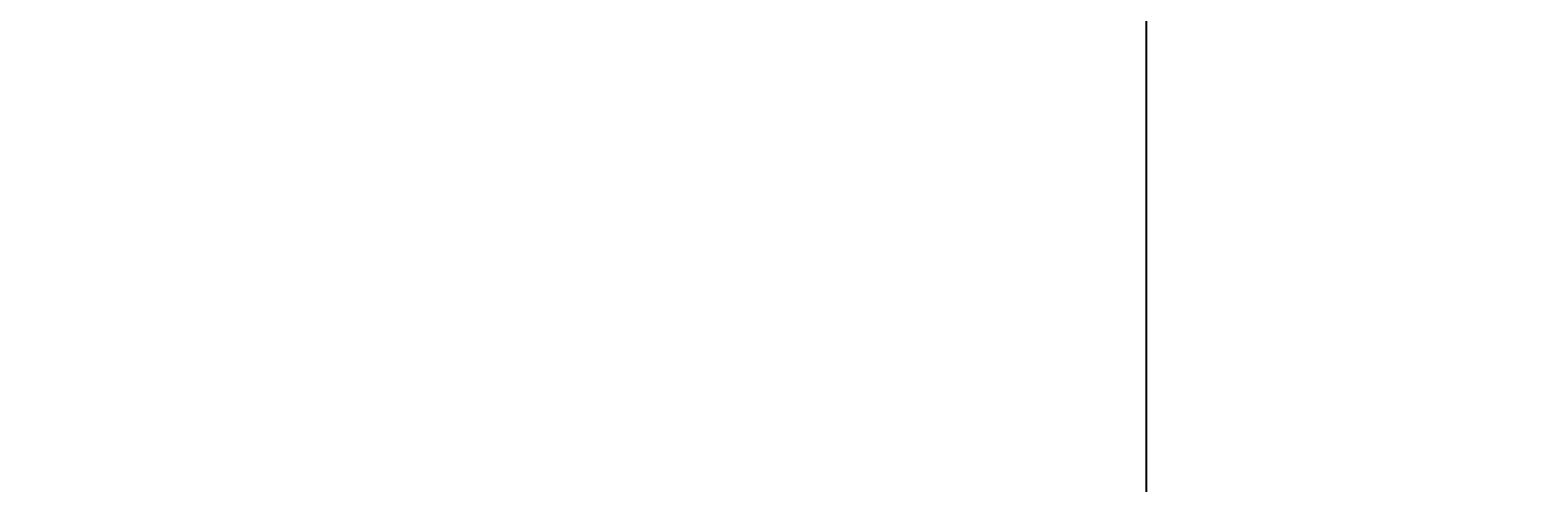
# Model space of a CAD drawing. Units: inches. Extents: x -301 to 715, y -607 to 364.
# Tile 15 of 141: x 18 to 59, y -499 to -486. Entities that reach past the tile are written whole.
import ezdxf

# ---------------------------------------------------------------- set-up
doc = ezdxf.new("R2010")
doc.units = ezdxf.units.IN
doc.header["$MEASUREMENT"] = 0
doc.layers.add('A-ANNO-DIMS', color=2, linetype='Continuous', lineweight=18)
doc.styles.get("Standard").update_dxf_attribs({"font": 'arial.ttf'})
doc.dimstyles.get("Standard").update_dxf_attribs({"dimtxt": 0.18, "dimasz": 0.18, "dimexe": 0.18, "dimexo": 0.0625, "dimgap": 0.09, "dimtad": 0, "dimtih": 1, "dimtoh": 1, "dimdec": 1, "dimzin": 0, "dimdsep": 46, "dimlunit": 4, "dimtxsty": 'Standard', "dimcen": 0.09, "dimclrd": 3, "dimclre": 4, "dimclrt": 6, "dimadec": 0, "dimazin": 0, "dimtfac": 1, "dimtdec": 1, "dimtofl": 0, "dimtmove": 0, "dimatfit": 3, "dimfxl": 1, "dimtfill": 2, "dimtfillclr": 51, "dimtolj": 1, "dimtzin": 0, "dimarcsym": 0})

# ---------------------------------------------------------------- blocks, each defined once
blk = doc.blocks.new('*D176')
at = {"layer": 'A-ANNO-DIMS', "color": 4, "lineweight": -2, "transparency": 16777216}
for p, q in [((148.28, -324.477), (215.605, -324.477)), ((-15.22, -540.477), (215.605, -540.477))]:
    blk.add_line(p, q, dxfattribs=at)
at = {"layer": 'A-ANNO-DIMS', "color": 3, "lineweight": -2, "transparency": 16777216}
for p, q in [((215.425, -324.657), (215.425, -432.296)), ((215.425, -540.297), (215.425, -432.659))]:
    blk.add_line(p, q, dxfattribs=at)
at = {"layer": 'A-ANNO-DIMS', "color": 3, "transparency": 16777216}
for points in [[(215.395, -324.657), (215.455, -324.657), (215.425, -324.477)], [(215.395, -540.297), (215.455, -540.297), (215.425, -540.477)]]:
    blk.add_solid(points, dxfattribs=at)
at = {"layer": 'Defpoints', "color": 0, "transparency": 16777216}
for p in [(148.218, -324.477), (-15.282, -540.477), (215.425, -540.477)]:
    blk.add_point(p, dxfattribs=at)
at = {"layer": 'A-ANNO-DIMS', "color": 6, "transparency": 16777216, "insert": (215.425, -432.477), "char_height": 0.18, "attachment_point": 5, "bg_fill": 1, "box_fill_scale": 1.25, "bg_fill_color": 51, "bg_fill_transparency": 0}
blk.add_mtext('\\A1;18\'-0"', dxfattribs=at)
blk = doc.blocks.new('*D181')
at = {"layer": 'A-ANNO-DIMS', "color": 4, "lineweight": -2, "transparency": 16777216}
for p, q in [((48.468, -433.54), (48.468, -573.809)), ((12.718, -463.54), (12.718, -573.809))]:
    blk.add_line(p, q, dxfattribs=at)
at = {"layer": 'A-ANNO-DIMS', "color": 3, "lineweight": -2, "transparency": 16777216}
for p, q in [((12.898, -573.629), (30.264, -573.629)), ((48.288, -573.629), (30.922, -573.629))]:
    blk.add_line(p, q, dxfattribs=at)
at = {"layer": 'A-ANNO-DIMS', "color": 3, "transparency": 16777216}
for points in [[(12.898, -573.599), (12.898, -573.659), (12.718, -573.629)], [(48.288, -573.599), (48.288, -573.659), (48.468, -573.629)]]:
    blk.add_solid(points, dxfattribs=at)
at = {"layer": 'Defpoints', "color": 0, "transparency": 16777216}
for p in [(48.468, -433.477), (12.718, -463.477), (48.468, -573.629)]:
    blk.add_point(p, dxfattribs=at)
at = {"layer": 'A-ANNO-DIMS', "color": 6, "transparency": 16777216, "insert": (30.593, -573.629), "char_height": 0.18, "attachment_point": 5, "bg_fill": 1, "box_fill_scale": 1.25, "bg_fill_color": 51, "bg_fill_transparency": 0}
blk.add_mtext('\\A1;3\'-0"', dxfattribs=at)
blk = doc.blocks.new('*D190')
at = {"layer": 'A-ANNO-DIMS', "color": 4, "lineweight": -2, "transparency": 16777216}
for p, q in [((129.193, -481.477), (-266.112, -481.477)), ((124.193, -511.477), (-266.112, -511.477))]:
    blk.add_line(p, q, dxfattribs=at)
at = {"layer": 'A-ANNO-DIMS', "color": 3, "lineweight": -2, "transparency": 16777216}
for p, q in [((-265.932, -481.657), (-265.932, -496.296)), ((-265.932, -511.297), (-265.932, -496.659))]:
    blk.add_line(p, q, dxfattribs=at)
at = {"layer": 'A-ANNO-DIMS', "color": 3, "transparency": 16777216}
for points in [[(-265.962, -481.657), (-265.902, -481.657), (-265.932, -481.477)], [(-265.962, -511.297), (-265.902, -511.297), (-265.932, -511.477)]]:
    blk.add_solid(points, dxfattribs=at)
at = {"layer": 'Defpoints', "color": 0, "transparency": 16777216}
for p in [(129.255, -481.477), (-265.932, -511.477), (124.255, -511.477)]:
    blk.add_point(p, dxfattribs=at)
at = {"layer": 'A-ANNO-DIMS', "color": 6, "transparency": 16777216, "insert": (-265.932, -496.477), "char_height": 0.18, "attachment_point": 5, "bg_fill": 1, "box_fill_scale": 1.25, "bg_fill_color": 51, "bg_fill_transparency": 0}
blk.add_mtext('\\A1;2\'-6"', dxfattribs=at)
blk = doc.blocks.new('*D191')
at = {"layer": 'A-ANNO-DIMS', "color": 4, "lineweight": -2, "transparency": 16777216}
for p, q in [((129.193, -481.477), (-266.112, -481.477)), ((114.193, -540.477), (-266.112, -540.477))]:
    blk.add_line(p, q, dxfattribs=at)
at = {"layer": 'A-ANNO-DIMS', "color": 3, "lineweight": -2, "transparency": 16777216}
for p, q in [((-265.932, -481.657), (-265.932, -510.797)), ((-265.932, -540.297), (-265.932, -511.158))]:
    blk.add_line(p, q, dxfattribs=at)
at = {"layer": 'A-ANNO-DIMS', "color": 3, "transparency": 16777216}
for points in [[(-265.962, -481.657), (-265.902, -481.657), (-265.932, -481.477)], [(-265.962, -540.297), (-265.902, -540.297), (-265.932, -540.477)]]:
    blk.add_solid(points, dxfattribs=at)
at = {"layer": 'Defpoints', "color": 0, "transparency": 16777216}
for p in [(129.255, -481.477), (-265.932, -540.477), (114.255, -540.477)]:
    blk.add_point(p, dxfattribs=at)
at = {"layer": 'A-ANNO-DIMS', "color": 6, "transparency": 16777216, "insert": (-265.932, -510.977), "char_height": 0.18, "attachment_point": 5, "bg_fill": 1, "box_fill_scale": 1.25, "bg_fill_color": 51, "bg_fill_transparency": 0}
blk.add_mtext('\\A1;4\'-11"', dxfattribs=at)

msp = doc.modelspace()

# ---------------------------------------------------------------- dimensions: what is measured, and where the dimension line sits
at = {"layer": 'A-ANNO-DIMS'}
for base, p1, p2, picture, middle in [((215.425, -540.477), (148.218, -324.477), (-15.282, -540.477), '*D176', (215.425, -432.477)), ((-265.932, -540.477), (129.255, -481.477), (114.255, -540.477), '*D191', (-265.932, -510.977)), ((-265.932, -511.477), (129.255, -481.477), (124.255, -511.477), '*D190', (-265.932, -496.477))]:
    dim = msp.add_linear_dim(base=base, p1=p1, p2=p2, angle=90, dimstyle='Standard', override={"dimdec": 1, "dimlfac": 1, "dimrnd": 0, "dimzin": 1, "dimdsep": 46, "dimlunit": 4, "dimfrac": 2}, dxfattribs=at)
    dim.commit()
    dim.dimension.update_dxf_attribs({"geometry": picture, "text_midpoint": middle})
dim = msp.add_linear_dim(base=(48.467984, -573.628877), p1=(12.717984, -463.47741), p2=(48.467984, -433.47741), dimstyle='Standard', override={"dimdec": 1, "dimlfac": 1, "dimrnd": 0, "dimzin": 1, "dimdsep": 46, "dimlunit": 4, "dimfrac": 2}, dxfattribs=at)
dim.commit()
dim.dimension.update_dxf_attribs({"geometry": '*D181', "text_midpoint": (30.592984, -573.628877)})

doc.saveas('drawing.dxf')
